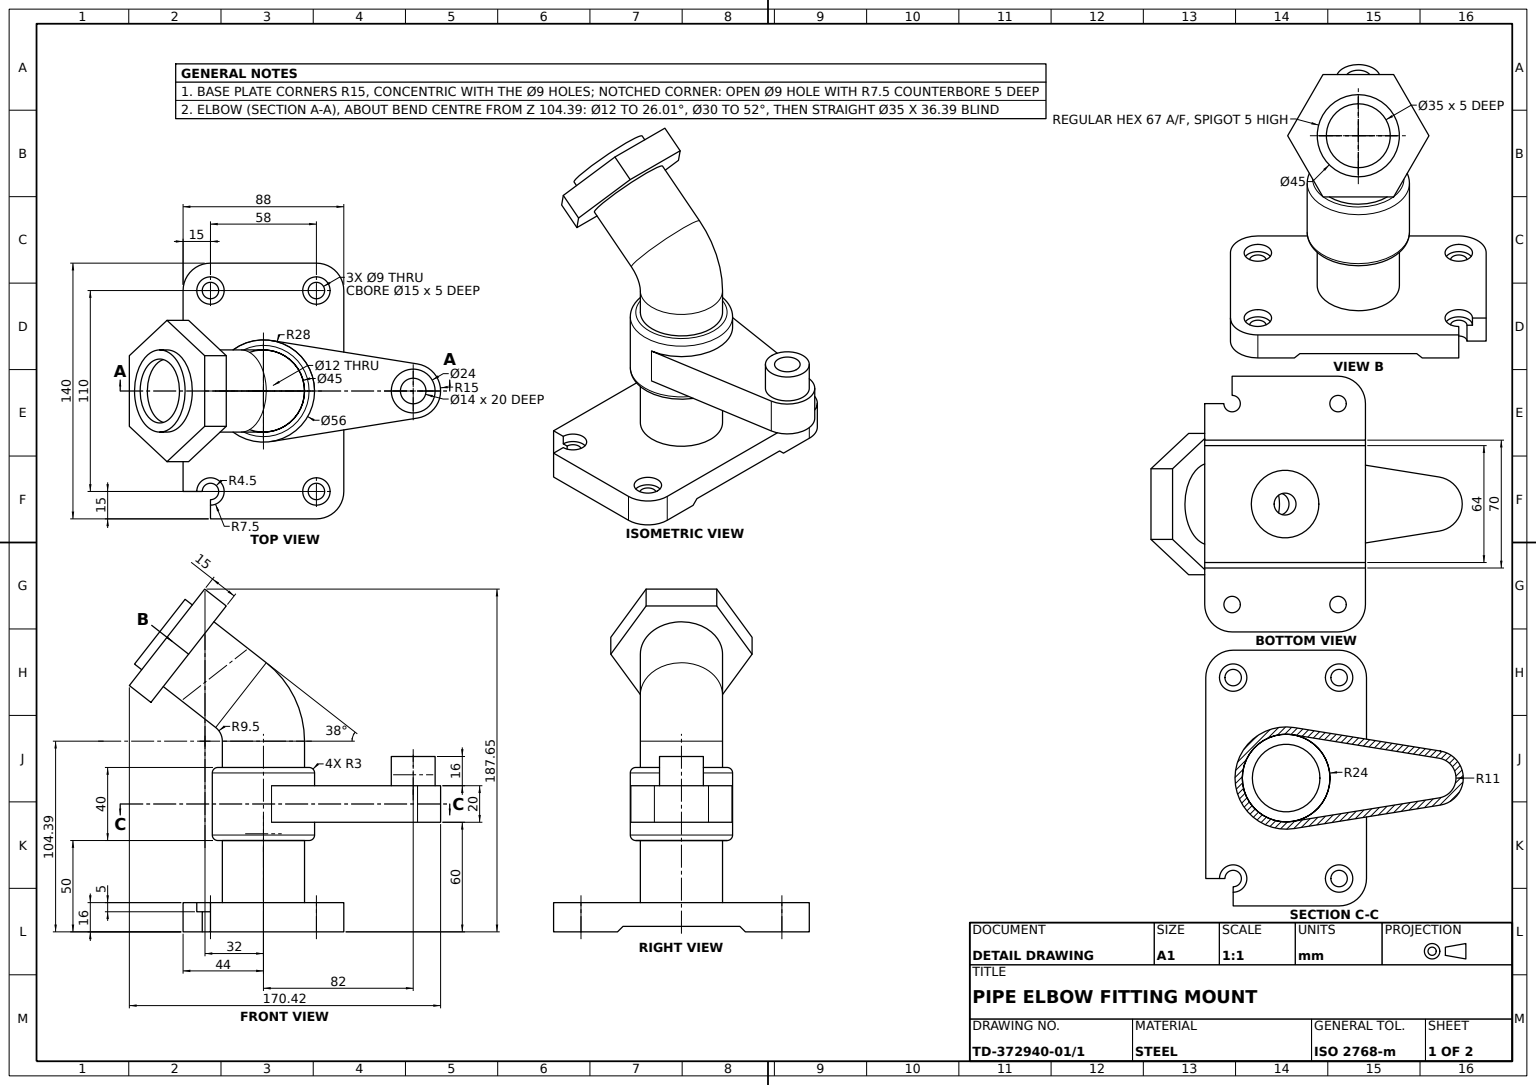
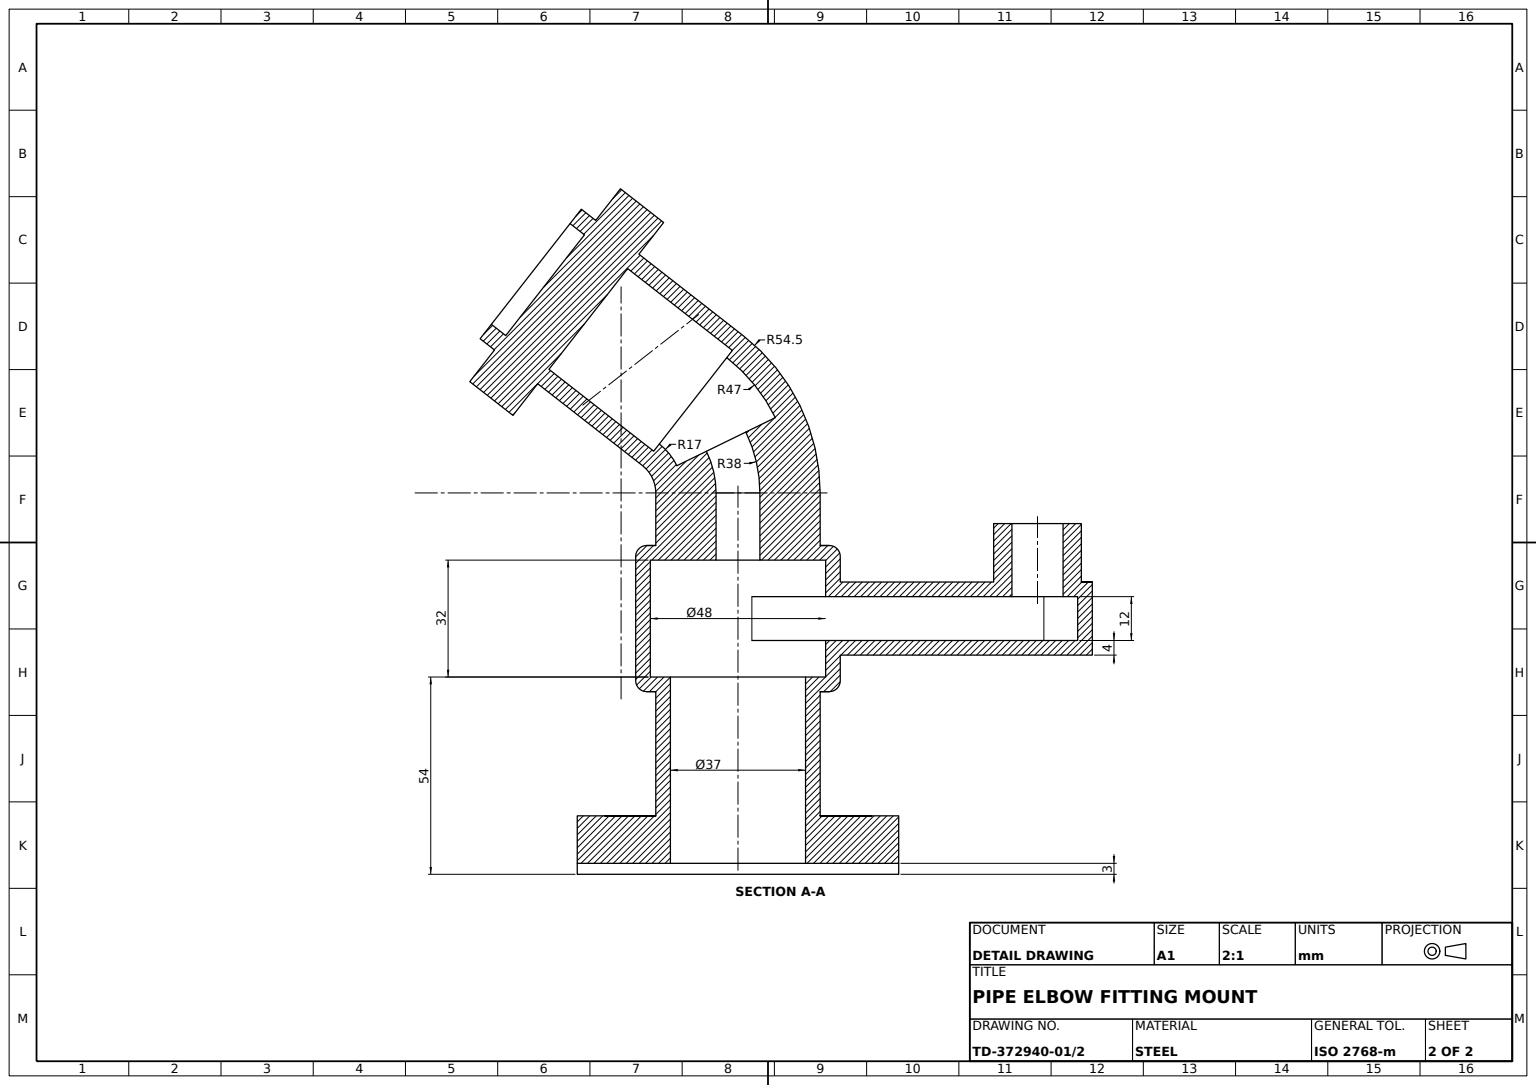
from build123d import *

# Parameters (mm, degrees)
BASE_PLATE_SKETCH_W                = 140
BASE_PLATE_SKETCH_H                = 88
BASE_PLATE_DEPTH                   = 16
BASE_PLATE_CORNER_FILLETS_R15_R    = 15
MOUNTING_HOLES_CBORE_9_D           = 9
MOUNTING_HOLES_CBORE_9_CBORE_D     = 15
MOUNTING_HOLES_CBORE_9_CBORE_DEPTH = 5
BASE_BORE_37_DEPTH                 = 85.214013086
BASE_BORE_37_DEPTH_BACK            = 16
BASE_BORE_SKETCH_37_R              = 18.5
PIPE_ELBOW_45_PROFILE_R            = 22.5
COLUMN_START                       = 50
COLUMN_SKETCH_56_R                 = 28
COLUMN_56_DEPTH                    = 40
PIPE_ELBOW_BORE_PROFILE_R          = 6
LUG_ARM_DEPTH                      = 10
LUG_START                          = 10
SKETCH24_3_R                       = 12
LUG_BOSS_DEPTH                     = 16
LUG_HOLE_REACH                     = 165.908
SKETCH24_4_R                       = 7
LUG_ARM_GROOVE_DEPTH               = 6
COLUMN_GROOVE_PROFILE_W            = 24
COLUMN_GROOVE_PROFILE_H            = 32
COLUMN_BORE_37_REACH               = 219.84
COLUMN_BORE_SKETCH_37_R            = 18.5
ELBOW_PROFILE_CUT_PROFILE_R        = 15
OUTLET_BORE_PROFILE_R              = 17.5
BASE_RECESS_REACH                  = 242.678
HEX_START                          = -5
HEX_OUTLET_67_DEPTH                = 15
BASE_EDGE_NOTCH_REACH              = 211.217
COLUMN_FILLET_R3_R                 = 3


with BuildPart() as part:
    # Base Plate Sketch → Base Plate (new body)
    with BuildSketch(Plane(origin=(0, 0, 0), x_dir=(1, 0, 0), z_dir=(0, 1, 0))):
        Rectangle(BASE_PLATE_SKETCH_W, BASE_PLATE_SKETCH_H)
    extrude(amount=BASE_PLATE_DEPTH)

    # Base Plate Corner Fillets R15
    base_plate_corner_fillets_r15_edges = [part.edges().sort_by_distance(p)[0] for p in [
        (70, 8, 44),
        (-70, 8, 44),
        (-70, 8, -44),
        (70, 8, -44),
    ]]
    fillet(base_plate_corner_fillets_r15_edges, radius=BASE_PLATE_CORNER_FILLETS_R15_R)

    # Mounting Holes CBore _9 (through all)
    with Locations(Plane(origin=(0, 16, 0), x_dir=(1, 0, 0), z_dir=(0, 1, 0))):
        with Locations((-55, 29), (-55, -29), (55, -29), (55, 29)):
            CounterBoreHole(MOUNTING_HOLES_CBORE_9_D / 2, MOUNTING_HOLES_CBORE_9_CBORE_D / 2, MOUNTING_HOLES_CBORE_9_CBORE_DEPTH)

    # Base Bore Sketch _37 → Base Bore _37 (cut, two sides: drawn at the far end of the back side and taken through both)
    with BuildSketch(Plane.XZ.offset(-BASE_BORE_37_DEPTH_BACK)):
        with Locations(Location((0, 0, 0), (0, 0, 270))):
            Circle(BASE_BORE_SKETCH_37_R)
    extrude(amount=BASE_BORE_37_DEPTH + BASE_BORE_37_DEPTH_BACK, mode=Mode.SUBTRACT)

    # Pipe Elbow _45: sweep along a path in Pipe Elbow Path
    with BuildLine(Plane(origin=(0, 0, 0), x_dir=(0, 0, -1), z_dir=(1, 0, 0))) as pipe_elbow_45_path:
        Line((0, 0), (0, 104.392557166))
        ThreePointArc((0, 104.392557166), (-3.238590518, 118.420433863), (-12.29883279, 129.608901281))
        Line((-12.29883279, 129.608901281), (-56.73677426, 164.327626223))
    # Pipe Elbow _45 profile (on start of the path) → Pipe Elbow _45 (sweep)
    with BuildSketch(Plane.ZX):
        Circle(PIPE_ELBOW_45_PROFILE_R)
    sweep(path=pipe_elbow_45_path.line)

    # Column Sketch _56 → Column _56 (add)
    with BuildSketch(Plane(origin=(0, 0, 0), x_dir=(1, 0, 0), z_dir=(0, 1, 0)).offset(COLUMN_START)):
        with Locations(Location((0, 0, 0), (0, 0, 270))):
            Circle(COLUMN_SKETCH_56_R)
    extrude(amount=COLUMN_56_DEPTH)

    # Pipe Elbow Bore: sweep along a path in Sketch8_4
    with BuildLine(Plane(origin=(0, 0, 0), x_dir=(0, 0, -1), z_dir=(1, 0, 0))) as pipe_elbow_bore_path:
        Line((0, 0), (0, 104.392557166))
        ThreePointArc((0, 104.392557166), (-3.238590518, 118.420433863), (-12.29883279, 129.608901281))
        Line((-12.29883279, 129.608901281), (-56.73677426, 164.327626223))
    # Pipe Elbow Bore profile (on start of the path) → Pipe Elbow Bore (sweep, cut)
    with BuildSketch(Plane.ZX):
        Circle(PIPE_ELBOW_BORE_PROFILE_R)
    sweep(path=pipe_elbow_bore_path.line, mode=Mode.SUBTRACT)

    # Lug Arm Sketch → Lug Arm (add, symmetric)
    with BuildSketch(Plane(origin=(0, 70, 0), x_dir=(1, 0, 0), z_dir=(0, 1, 0))):
        with BuildLine():
            Line((27.6458869, 4.43902439), (14.810296553, 84.37804878))
            ThreePointArc((14.810296553, 84.37804878), (0, 97), (-14.810296553, 84.37804878))
            Line((-14.810296553, 84.37804878), (-27.6458869, 4.43902439))
            ThreePointArc((-27.6458869, 4.43902439), (0, 28), (27.6458869, 4.43902439))
        make_face()
    extrude(amount=LUG_ARM_DEPTH, both=True)

    # Sketch24_3 → Lug Boss (add)
    with BuildSketch(Plane(origin=(0, 70, 0), x_dir=(1, 0, 0), z_dir=(0, 1, 0)).offset(LUG_START)):
        with Locations(Location((0, 82, 0), (0, 0, 270))):
            Circle(SKETCH24_3_R)
    extrude(amount=LUG_BOSS_DEPTH)

    # Sketch24_4 → Lug Hole (cut, up to next)
    with BuildSketch(Plane(origin=(0, 70, 0), x_dir=(1, 0, 0), z_dir=(0, 1, 0)), mode=Mode.PRIVATE) as lug_hole_sk1:
        with Locations(Location((0, 82, 0), (0, 0, 270))):
            Circle(SKETCH24_4_R)
    lug_hole_tool1 = extrude(lug_hole_sk1.sketch, amount=LUG_HOLE_REACH, mode=Mode.PRIVATE) & part.part
    add(lug_hole_tool1.solids().sort_by_distance((0, 70, -82))[0], mode=Mode.SUBTRACT)

    # Lug Arm Groove Sketch → Lug Arm Groove (cut, symmetric)
    with BuildSketch(Plane(origin=(0, 70, 0), x_dir=(1, 0, 0), z_dir=(0, 1, 0))):
        with BuildLine():
            Line((23.696474485, 3.804878049), (10.860884139, 83.743902439))
            ThreePointArc((10.860884139, 83.743902439), (0, 93), (-10.860884139, 83.743902439))
            Line((-10.860884139, 83.743902439), (-23.696474485, 3.804878049))
            ThreePointArc((-23.696474485, 3.804878049), (0, 24), (23.696474485, 3.804878049))
        make_face()
    extrude(amount=LUG_ARM_GROOVE_DEPTH, both=True, mode=Mode.SUBTRACT)

    # Column Groove Profile → Column Groove (revolve, cut)
    with BuildSketch(Plane(origin=(0, 0, 0), x_dir=(0, 0, -1), z_dir=(1, 0, 0)), mode=Mode.PRIVATE) as column_groove_sk:
        with Locations((-12, 70)):
            Rectangle(COLUMN_GROOVE_PROFILE_W, COLUMN_GROOVE_PROFILE_H)
    revolve(column_groove_sk.sketch.rotate(Axis((0, 0, 0), (0, 1, 0)), 180), axis=Axis((0, 0, 0), (0, 1, 0)), mode=Mode.SUBTRACT)

    # Column Bore Sketch _37 → Column Bore _37 (cut, up to next)
    with BuildSketch(Plane.XZ, mode=Mode.PRIVATE) as column_bore_37_sk1:
        with Locations(Location((0, 0, 0), (0, 0, 270))):
            Circle(COLUMN_BORE_SKETCH_37_R)
    column_bore_37_tool1 = extrude(column_bore_37_sk1.sketch, amount=-COLUMN_BORE_37_REACH, mode=Mode.PRIVATE) & part.part
    add(column_bore_37_tool1.solids().sort_by_distance((0, 0, 0))[0], mode=Mode.SUBTRACT)

    # Elbow Profile Cut: sweep along a path in Elbow Profile Cut Sketch
    with BuildLine(Plane(origin=(0, 0, 0), x_dir=(0, 0, -1), z_dir=(1, 0, 0))) as elbow_profile_cut_path:
        ThreePointArc((-3.240841211, 118.425047527), (-7.132944581, 124.532804305), (-12.29883279, 129.608901281))
    # Elbow Profile Cut profile (on start of the path) → Elbow Profile Cut (sweep, cut)
    with BuildSketch(Plane(origin=(0, 118.425047527, 3.240841211), x_dir=(0, -0.4385153237962811, 0.898723712158438), z_dir=(0, 0.898723712158438, 0.4385153237962811))):
        Circle(ELBOW_PROFILE_CUT_PROFILE_R)
    sweep(path=elbow_profile_cut_path.line, mode=Mode.SUBTRACT)

    # Outlet Bore: sweep along a path in Outlet Bore Path
    with BuildLine(Plane(origin=(0, 0, 0), x_dir=(0, 0, -1), z_dir=(1, 0, 0))) as outlet_bore_path:
        Line((-12.29883279, 129.608901281), (-56.73677426, 164.327626223))
    # Outlet Bore profile (on start of the path) → Outlet Bore (sweep, cut)
    with BuildSketch(Plane(origin=(0, 129.608901281, 12.29883279), x_dir=(0, 0.7880107536067169, -0.6156614753256648), z_dir=(0, 0.6156614753256648, 0.7880107536067169))):
        Circle(OUTLET_BORE_PROFILE_R)
    sweep(path=outlet_bore_path.line, mode=Mode.SUBTRACT)

    # Base Recess Sketch → Base Recess (cut, up to next)
    with BuildSketch(Plane.XY.offset(44), mode=Mode.PRIVATE) as base_recess_sk1:
        Polygon((35, 0), (-35, 0), (-32, 3), (32, 3), align=None)
    base_recess_tool1 = extrude(base_recess_sk1.sketch, amount=-BASE_RECESS_REACH, mode=Mode.PRIVATE) & part.part
    add(base_recess_tool1.solids().sort_by_distance((0, 1.477612, 44))[0], mode=Mode.SUBTRACT)

    # Hex Outlet Sketch 67 → Hex Outlet 67 (add)
    with BuildSketch(Plane(origin=(0, 89.812312487, 114.954517836), x_dir=(1, 0, 0), z_dir=(0, 0.6156614753256595, 0.7880107536067211)).offset(HEX_START)):
        Polygon((38.682468036, 94.561290433), (19.341234018, 128.061290433), (-19.341234018, 128.061290433), (-38.682468036, 94.561290433), (-19.341234018, 61.061290433), (19.341234018, 61.061290433), align=None)
    extrude(amount=-HEX_OUTLET_67_DEPTH)

    # Base Edge Notch Sketch → Base Edge Notch (cut, up to next)
    with BuildSketch(Plane(origin=(0, 16, 0), x_dir=(1, 0, 0), z_dir=(0, 1, 0)), mode=Mode.PRIVATE) as base_edge_notch_sk1:
        with BuildLine():
            Line((55, -29), (70, -29))
            ThreePointArc((70, -29), (65.606601718, -39.606601718), (55, -44))
            Line((55, -44), (55, -29))
        make_face()
    base_edge_notch_tool1 = extrude(base_edge_notch_sk1.sketch, amount=-BASE_EDGE_NOTCH_REACH, mode=Mode.PRIVATE) & part.part
    add(base_edge_notch_tool1.solids().sort_by_distance((61.366198, 16, 35.366198))[0], mode=Mode.SUBTRACT)

    # Column Fillet R3
    column_fillet_r3_edges = [part.edges().sort_by_distance(p)[0] for p in [
        (0, 50, -28),
        (0, 90, -28),
    ]]
    fillet(column_fillet_r3_edges, radius=COLUMN_FILLET_R3_R)


solid = part.part
